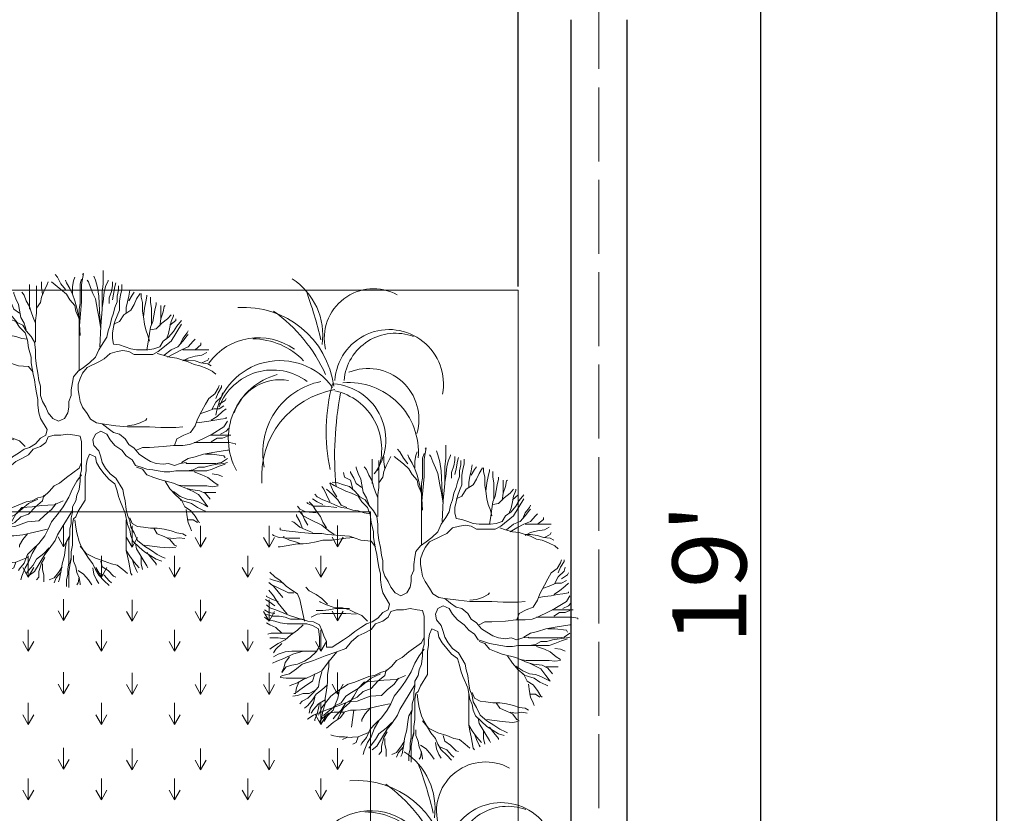
# Model space of a CAD drawing. Units: millimetres. Extents: x 595116 to 630915, y 909473 to 920225.
# Tile 111 of 134: x 629744 to 629904, y 919217 to 919346. Entities that reach past the tile are written whole.
import ezdxf

# ---------------------------------------------------------------- set-up
doc = ezdxf.new("R2010")
doc.units = ezdxf.units.MM
doc.linetypes.add('ACAD_ISO02W100', pattern=[15, 12, -3])
for name, color, linetype, lineweight in [('C-PROP', 7, 'Continuous', 25), ('C-PROP-REF', 240, 'ACAD_ISO02W100', 13), ('Dimension', 3, 'Continuous', 18), ('L-PLNT', 85, 'Continuous', 13)]:
    doc.layers.add(name, color=color, linetype=linetype, lineweight=lineweight)
doc.styles.get("Standard").update_dxf_attribs({"font": 'arial.ttf'})
doc.dimstyles.new('ISO-25', dxfattribs={"dimtxt": 9, "dimasz": 6, "dimexe": 1.25, "dimexo": 0.625, "dimtad": 1, "dimlunit": 4, "dimtxsty": 'Standard', "dimcen": 2.5, "dimadec": 0, "dimazin": 0, "dimtfac": 1, "dimtmove": 0, "dimatfit": 3, "dimfxl": 1, "dimarcsym": 0})

# ---------------------------------------------------------------- blocks, each defined once
blk = doc.blocks.new('tree')
for centre, radius, start, end in [((629595.141, 919296.95), 5.184, 352.03203, 57.07138), ((629569.835, 919289.496), 31.168, 13.14902, 20.50764), ((629604.232, 919296.737), 3.791, 61.13475, 193.10801), ((629594.259, 919292.132), 6.965, 7.40006, 94.00585), ((629589.446, 919288.922), 12.167, 24.2477, 54.37264), ((629605.429, 919293.205), 4.185, 348.99772, 176.315), ((629605.915, 919293.144), 3.963, 69.38448, 175.23101), ((629595.377, 919292.044), 4.722, 54.24842, 144.21671), ((629594.88, 919291.171), 5.506, 43.86717, 89.48049), ((629597.025, 919289.989), 5.01, 36.05808, 170.65417), ((629596.464, 919289.874), 4.4, 52.90738, 159.34709), ((629598.153, 919288.998), 5.103, 105.35763, 208.89728), ((629603.809, 919290.469), 3.92, 343.88599, 112.26625), ((629597.068, 919289.758), 3.768, 80.48165, 161.06642), ((629601.247, 919287.941), 5.545, 101.04188, 191.86923), ((629614.329, 919289.554), 13.748, 164.59254, 192.32305), ((629600.849, 919288.894), 4.324, 322.54615, 85.80496), ((629602.329, 919287.957), 5.355, 355.21411, 94.82173), ((629602.391, 919286.088), 6.769, 99.68104, 184.5451), ((629626.813, 919287.645), 25.579, 169.07531, 185.28887), ((629600.275, 919288.191), 4.585, 338.7925, 77.69211)]:
    blk.add_arc(centre, radius, start, end)
blk = doc.blocks.new('A$C143125F4')
for p, q in [((2.883, 4.834), (2.883, 5.044)), ((1.898, 4.776), (1.898, 4.865)), ((1.991, 4.82), (2.008, 4.865)), ((2.21, 4.744), (2.062, 4.865)), ((2.155, 4.937), (2.117, 4.982)), ((2.21, 4.834), (2.155, 4.937)), ((2.298, 4.847), (2.281, 4.892)), ((2.391, 4.789), (2.407, 4.879)), ((2.407, 4.879), (2.429, 4.937)), ((2.516, 4.834), (2.538, 4.91)), ((2.538, 4.82), (2.571, 5)), ((2.571, 5), (2.555, 4.982)), ((2.648, 4.865), (2.626, 4.892)), ((2.681, 4.776), (2.648, 4.865)), ((2.757, 4.892), (2.735, 4.955)), ((2.79, 4.776), (2.757, 4.892)), ((2.921, 4.789), (2.96, 4.879)), ((2.96, 4.879), (2.96, 4.892)), ((3.031, 4.802), (3.031, 4.865)), ((1.461, 4.681), (1.461, 4.699)), ((1.625, 4.655), (1.586, 4.699)), ((1.712, 4.431), (1.712, 4.82)), ((1.822, 4.368), (1.822, 4.802)), ((1.915, 4.668), (1.898, 4.776)), ((1.898, 4.623), (1.937, 4.713)), ((1.937, 4.713), (1.991, 4.82)), ((2.281, 4.744), (2.21, 4.834)), ((2.298, 4.668), (2.21, 4.744)), ((2.352, 4.758), (2.298, 4.847)), ((2.391, 4.668), (2.352, 4.758)), ((2.391, 4.681), (2.391, 4.789)), ((2.516, 4.52), (2.516, 4.834)), ((2.538, 4.547), (2.538, 4.82)), ((2.719, 4.681), (2.681, 4.776)), ((2.812, 4.637), (2.79, 4.776)), ((2.867, 4.699), (2.883, 4.834)), ((2.867, 4.431), (2.867, 4.699)), ((2.883, 4.547), (2.899, 4.699)), ((2.899, 4.699), (2.921, 4.789)), ((2.976, 4.61), (3.014, 4.713)), ((3.014, 4.713), (3.031, 4.802)), ((3.047, 4.668), (3.069, 4.789)), ((3.069, 4.789), (3.085, 4.847)), ((3.102, 4.637), (3.124, 4.731)), ((3.124, 4.731), (3.124, 4.802)), ((3.156, 4.655), (3.178, 4.744)), ((3.178, 4.744), (3.178, 4.82)), ((3.288, 4.637), (3.304, 4.731)), ((3.342, 4.655), (3.375, 4.699)), ((1.275, 4.534), (1.258, 4.61)), ((1.368, 4.61), (1.368, 4.623)), ((1.422, 4.52), (1.368, 4.61)), ((1.493, 4.592), (1.461, 4.681)), ((1.532, 4.502), (1.493, 4.592)), ((1.658, 4.565), (1.625, 4.655)), ((1.712, 4.475), (1.658, 4.565)), ((1.882, 4.534), (1.898, 4.623)), ((2.352, 4.578), (2.298, 4.668)), ((2.429, 4.489), (2.352, 4.578)), ((2.429, 4.565), (2.391, 4.668)), ((2.462, 4.444), (2.429, 4.565)), ((2.5, 4.099), (2.538, 4.547)), ((2.757, 4.592), (2.719, 4.681)), ((2.79, 4.413), (2.757, 4.592)), ((2.828, 4.296), (2.812, 4.637)), ((2.867, 4.457), (2.883, 4.547)), ((2.976, 4.52), (2.976, 4.61)), ((3.031, 4.578), (3.047, 4.668)), ((3.069, 4.457), (3.102, 4.547)), ((3.102, 4.547), (3.102, 4.637)), ((3.14, 4.565), (3.156, 4.655)), ((3.14, 4.413), (3.14, 4.565)), ((3.249, 4.457), (3.266, 4.547)), ((3.266, 4.547), (3.288, 4.637)), ((3.288, 4.565), (3.342, 4.655)), ((3.375, 4.502), (3.414, 4.592)), ((3.414, 4.592), (3.468, 4.681)), ((3.485, 4.623), (3.485, 4.681)), ((3.507, 4.534), (3.485, 4.623)), ((3.539, 4.444), (3.561, 4.547)), ((3.561, 4.547), (3.578, 4.637)), ((3.578, 4.637), (3.578, 4.655)), ((3.632, 4.534), (3.632, 4.623)), ((0.946, 4.341), (0.914, 4.386)), ((1.111, 4.399), (1.039, 4.444)), ((1.056, 4.399), (1.039, 4.431)), ((1.094, 4.31), (1.056, 4.399)), ((1.078, 4.457), (1.165, 4.444)), ((1.297, 4.31), (1.111, 4.399)), ((1.165, 4.444), (1.258, 4.413)), ((1.258, 4.413), (1.351, 4.386)), ((1.368, 4.489), (1.275, 4.534)), ((1.351, 4.386), (1.439, 4.31)), ((1.406, 4.341), (1.368, 4.489)), ((1.461, 4.431), (1.422, 4.52)), ((1.548, 4.368), (1.461, 4.431)), ((1.548, 4.413), (1.532, 4.502)), ((1.57, 4.296), (1.548, 4.413)), ((1.734, 4.386), (1.712, 4.475)), ((1.767, 4.296), (1.734, 4.386)), ((1.822, 4.444), (1.882, 4.534)), ((2.445, 4.399), (2.429, 4.489)), ((2.5, 4.278), (2.445, 4.399)), ((2.484, 4.354), (2.462, 4.444)), ((2.5, 4.431), (2.516, 4.52)), ((2.5, 3.458), (2.5, 4.431)), ((2.812, 4.31), (2.79, 4.413)), ((2.845, 4.162), (2.867, 4.431)), ((3.047, 4.368), (3.069, 4.457)), ((3.102, 4.323), (3.14, 4.413)), ((3.211, 4.341), (3.321, 4.413)), ((3.249, 4.368), (3.249, 4.457)), ((3.321, 4.413), (3.375, 4.502)), ((3.507, 4.399), (3.507, 4.534)), ((3.523, 4.31), (3.507, 4.399)), ((3.523, 4.31), (3.539, 4.444)), ((3.649, 4.444), (3.632, 4.534)), ((3.649, 4.189), (3.649, 4.444)), ((3.671, 4.233), (3.704, 4.413)), ((3.704, 4.413), (3.725, 4.502)), ((3.725, 4.502), (3.725, 4.534)), ((3.797, 4.278), (3.797, 4.489)), ((3.797, 4.278), (3.835, 4.386)), ((3.835, 4.386), (3.851, 4.475)), ((3.851, 4.475), (3.868, 4.489)), ((0.837, 4.22), (0.804, 4.265)), ((0.985, 4.251), (0.946, 4.341)), ((1.078, 4.265), (0.985, 4.341)), ((1.039, 4.144), (0.985, 4.251)), ((1.165, 4.175), (1.078, 4.265)), ((1.149, 4.22), (1.094, 4.31)), ((1.384, 4.278), (1.297, 4.31)), ((1.493, 4.233), (1.384, 4.278)), ((1.439, 4.31), (1.515, 4.22)), ((1.548, 4.144), (1.493, 4.233)), ((1.625, 4.207), (1.57, 4.296)), ((1.805, 4.207), (1.767, 4.296)), ((1.805, 4.251), (1.822, 4.368)), ((1.805, 3.906), (1.805, 4.251)), ((2.5, 4.265), (2.484, 4.354)), ((2.516, 4.009), (2.5, 4.278)), ((2.828, 4.22), (2.812, 4.31)), ((2.845, 4.207), (2.828, 4.296)), ((2.992, 4.175), (3.014, 4.278)), ((3.014, 4.278), (3.047, 4.368)), ((3.047, 4.189), (3.14, 4.233)), ((3.047, 4.144), (3.069, 4.233)), ((3.069, 4.233), (3.102, 4.323)), ((3.14, 4.233), (3.211, 4.341)), ((3.539, 4.189), (3.523, 4.31)), ((3.632, 4.144), (3.671, 4.233)), ((3.78, 4.162), (3.797, 4.278)), ((3.813, 4.207), (3.906, 4.278)), ((3.906, 4.278), (3.961, 4.341)), ((3.944, 4.175), (4.037, 4.251)), ((3.944, 4.144), (3.961, 4.233)), ((3.961, 4.233), (3.999, 4.323)), ((3.999, 4.323), (3.999, 4.341)), ((4.037, 4.251), (4.037, 4.278)), ((4.125, 4.251), (4.054, 4.162)), ((0.689, 4.117), (0.673, 4.13)), ((0.782, 4.072), (0.689, 4.117)), ((0.766, 4.086), (0.711, 4.144)), ((0.837, 4.144), (0.766, 4.189)), ((0.821, 3.996), (0.766, 4.086)), ((0.93, 4.175), (0.837, 4.22)), ((0.93, 4.099), (0.837, 4.144)), ((1.039, 4.13), (0.93, 4.175)), ((1.132, 4.086), (1.039, 4.13)), ((1.22, 4.054), (1.132, 4.086)), ((1.22, 4.086), (1.165, 4.175)), ((1.313, 4.054), (1.22, 4.086)), ((1.515, 4.22), (1.603, 4.175)), ((1.641, 4.054), (1.548, 4.144)), ((1.603, 4.175), (1.658, 4.086)), ((1.658, 4.099), (1.625, 4.207)), ((1.658, 4.086), (1.734, 3.996)), ((2.5, 3.996), (2.5, 4.099)), ((2.845, 4.117), (2.828, 4.22)), ((2.828, 3.83), (2.845, 4.162)), ((2.938, 3.983), (2.96, 4.086)), ((2.96, 4.086), (2.992, 4.175)), ((3.031, 4.054), (3.047, 4.144)), ((3.561, 4.099), (3.539, 4.189)), ((3.594, 4.009), (3.561, 4.099)), ((3.594, 3.875), (3.632, 4.144)), ((3.632, 4.099), (3.725, 4.117)), ((3.725, 4.117), (3.813, 4.207)), ((3.922, 4.041), (3.944, 4.144)), ((3.961, 3.92), (4.125, 4.189)), ((4.054, 4.162), (3.999, 4.072)), ((4.218, 4.054), (4.234, 4.086)), ((0.509, 3.92), (0.509, 3.938)), ((0.563, 3.83), (0.509, 3.92)), ((0.563, 4.027), (0.525, 4.072)), ((0.602, 3.951), (0.547, 3.996)), ((0.656, 3.983), (0.563, 4.027)), ((0.618, 3.92), (0.563, 3.983)), ((0.635, 3.862), (0.602, 3.951)), ((0.728, 3.862), (0.618, 3.92)), ((0.821, 3.965), (0.656, 3.983)), ((0.968, 4.072), (0.782, 4.072)), ((0.892, 3.906), (0.821, 3.996)), ((1.149, 4.054), (0.968, 4.072)), ((1.313, 4.041), (1.22, 4.054)), ((1.406, 4.009), (1.313, 4.041)), ((1.493, 3.996), (1.406, 4.009)), ((1.586, 3.965), (1.493, 3.996)), ((1.679, 3.951), (1.586, 3.965)), ((1.679, 3.938), (1.641, 4.054)), ((1.696, 3.817), (1.679, 3.938)), ((1.734, 3.996), (1.789, 3.906)), ((2.883, 3.893), (2.938, 3.983)), ((3.031, 3.965), (3.031, 4.054)), ((3.047, 3.875), (3.031, 3.965)), ((3.616, 3.92), (3.594, 4.009)), ((3.758, 3.754), (3.961, 3.92)), ((3.835, 3.92), (3.78, 3.83)), ((3.922, 3.983), (3.835, 3.92)), ((3.89, 3.951), (3.922, 4.041)), ((3.999, 4.072), (3.922, 3.983)), ((4.07, 3.83), (4.147, 3.92)), ((4.108, 3.875), (4.147, 3.965)), ((4.147, 3.965), (4.218, 4.054)), ((4.147, 3.92), (4.218, 4.009)), ((4.218, 4.009), (4.234, 4.027)), ((4.234, 3.83), (4.311, 3.92)), ((4.311, 3.92), (4.344, 3.951)), ((0.47, 3.817), (0.438, 3.83)), ((0.563, 3.741), (0.47, 3.817)), ((0.602, 3.727), (0.563, 3.83)), ((0.689, 3.772), (0.635, 3.862)), ((0.914, 3.772), (0.728, 3.862)), ((0.93, 3.817), (0.892, 3.906)), ((1.023, 3.682), (0.914, 3.772)), ((0.985, 3.727), (0.93, 3.817)), ((1.734, 3.665), (1.696, 3.817)), ((1.789, 3.906), (1.805, 3.785)), ((1.805, 3.785), (1.805, 3.651)), ((2.757, 3.665), (2.812, 3.785)), ((2.812, 3.785), (2.883, 3.893)), ((3.14, 3.862), (3.047, 3.875)), ((3.102, 3.754), (3.195, 3.772)), ((3.233, 3.83), (3.14, 3.862)), ((3.195, 3.772), (3.288, 3.754)), ((3.321, 3.799), (3.233, 3.83)), ((3.414, 3.785), (3.321, 3.799)), ((3.594, 3.785), (3.414, 3.785)), ((3.578, 3.785), (3.594, 3.875)), ((3.687, 3.799), (3.594, 3.785)), ((3.78, 3.83), (3.687, 3.799)), ((3.851, 3.696), (3.961, 3.785)), ((3.961, 3.785), (4.07, 3.83)), ((4.015, 3.727), (4.125, 3.785)), ((4.125, 3.785), (4.234, 3.83)), ((4.147, 3.785), (4.562, 3.785)), ((4.344, 3.785), (4.437, 3.862)), ((4.437, 3.862), (4.437, 3.893)), ((0.142, 3.606), (0.126, 3.62)), ((0.235, 3.575), (0.142, 3.606)), ((0.252, 3.696), (0.252, 3.727)), ((0.345, 3.682), (0.252, 3.696)), ((0.492, 3.665), (0.345, 3.682)), ((0.58, 3.651), (0.492, 3.665)), ((0.656, 3.696), (0.563, 3.741)), ((0.766, 3.638), (0.58, 3.651)), ((0.766, 3.651), (0.656, 3.696)), ((0.914, 3.638), (0.766, 3.638)), ((1.001, 3.62), (0.914, 3.638)), ((1.204, 3.606), (1.001, 3.62)), ((1.111, 3.62), (1.023, 3.682)), ((1.351, 3.593), (1.204, 3.606)), ((1.734, 3.575), (1.734, 3.665)), ((1.805, 3.651), (1.822, 3.53)), ((2.664, 3.575), (2.757, 3.665)), ((2.812, 3.593), (2.899, 3.638)), ((2.899, 3.638), (2.992, 3.727)), ((2.992, 3.727), (3.102, 3.754)), ((3.288, 3.754), (3.375, 3.709)), ((3.375, 3.709), (3.671, 3.709)), ((3.671, 3.709), (3.758, 3.754)), ((3.742, 3.727), (3.835, 3.696)), ((3.835, 3.696), (3.944, 3.665)), ((3.906, 3.665), (4.015, 3.727)), ((3.944, 3.665), (4.054, 3.651)), ((4.054, 3.651), (4.147, 3.62)), ((4.147, 3.606), (4.234, 3.651)), ((4.147, 3.62), (4.234, 3.593)), ((4.147, 3.62), (4.234, 3.62)), ((4.234, 3.651), (4.344, 3.682)), ((4.234, 3.62), (4.344, 3.606)), ((4.344, 3.682), (4.453, 3.696)), ((4.344, 3.606), (4.437, 3.575)), ((4.453, 3.696), (4.53, 3.741)), ((4.453, 3.575), (4.546, 3.62)), ((4.546, 3.62), (4.562, 3.651)), ((0.383, 3.561), (0.235, 3.575)), ((0.306, 3.575), (0.306, 3.593)), ((0.399, 3.53), (0.306, 3.575)), ((0.438, 3.458), (0.345, 3.441)), ((0.563, 3.561), (0.383, 3.561)), ((0.492, 3.503), (0.399, 3.53)), ((0.525, 3.472), (0.438, 3.458)), ((0.58, 3.472), (0.492, 3.503)), ((0.618, 3.472), (0.525, 3.472)), ((0.711, 3.485), (0.618, 3.472)), ((0.821, 3.503), (0.711, 3.485)), ((0.93, 3.53), (0.821, 3.503)), ((1.078, 3.53), (0.93, 3.53)), ((1.297, 3.561), (1.078, 3.53)), ((1.422, 3.575), (1.297, 3.561)), ((1.532, 3.53), (1.351, 3.593)), ((1.696, 3.517), (1.532, 3.53)), ((1.767, 3.427), (1.696, 3.517)), ((1.767, 3.396), (1.734, 3.575)), ((1.822, 3.53), (1.844, 3.414)), ((2.484, 3.441), (2.571, 3.503)), ((2.555, 3.414), (2.626, 3.503)), ((2.571, 3.503), (2.664, 3.575)), ((2.626, 3.503), (2.812, 3.593)), ((4.234, 3.593), (4.327, 3.548)), ((4.327, 3.548), (4.42, 3.53)), ((4.42, 3.53), (4.53, 3.485)), ((4.437, 3.575), (4.546, 3.561)), ((4.53, 3.485), (4.617, 3.441)), ((4.546, 3.561), (4.601, 3.53)), ((0.252, 3.427), (0.219, 3.427)), ((0.345, 3.441), (0.252, 3.427)), ((1.789, 3.306), (1.767, 3.396)), ((1.805, 3.19), (1.789, 3.306)), ((1.844, 3.414), (1.86, 3.293)), ((1.86, 3.293), (1.882, 3.203)), ((2.391, 3.261), (2.407, 3.351)), ((2.407, 3.351), (2.484, 3.441)), ((2.484, 3.234), (2.516, 3.324)), ((2.516, 3.324), (2.555, 3.414)), ((4.617, 3.441), (4.672, 3.396)), ((1.822, 3.1), (1.805, 3.19)), ((1.882, 3.203), (1.882, 3.055)), ((2.374, 3.145), (2.391, 3.261)), ((2.374, 3.055), (2.374, 3.145)), ((2.484, 3.145), (2.484, 3.234)), ((2.5, 3.055), (2.484, 3.145)), ((4.655, 3.082), (4.71, 3.172)), ((4.71, 3.172), (4.727, 3.217)), ((4.71, 3.1), (4.765, 3.19)), ((4.765, 3.19), (4.765, 3.217)), ((0.164, 2.948), (0.088, 3.024)), ((1.844, 2.993), (1.822, 3.1)), ((1.844, 2.903), (1.844, 2.993)), ((1.882, 3.055), (1.915, 2.961)), ((2.336, 2.961), (2.374, 3.055)), ((2.516, 2.961), (2.5, 3.055)), ((4.508, 2.916), (4.562, 3.01)), ((4.562, 3.01), (4.655, 3.082)), ((4.672, 3.01), (4.71, 3.1)), ((4.672, 2.948), (4.765, 3.037)), ((4.727, 2.916), (4.82, 2.979)), ((4.765, 3.037), (4.781, 3.1)), ((4.82, 2.979), (4.836, 3.01)), ((0.142, 2.8), (0.071, 2.858)), ((0.109, 2.827), (0.071, 2.858)), ((0.126, 2.903), (0.088, 2.916)), ((0.197, 2.782), (0.109, 2.827)), ((0.219, 2.872), (0.126, 2.903)), ((0.252, 2.89), (0.164, 2.948)), ((0.306, 2.845), (0.219, 2.872)), ((0.345, 2.8), (0.252, 2.89)), ((1.86, 2.782), (1.844, 2.903)), ((1.915, 2.961), (1.969, 2.872)), ((1.969, 2.872), (2.008, 2.782)), ((2.32, 2.782), (2.336, 2.872)), ((2.336, 2.872), (2.336, 2.961)), ((2.555, 2.872), (2.516, 2.961)), ((2.626, 2.769), (2.555, 2.872)), ((4.453, 2.813), (4.508, 2.916)), ((4.53, 2.8), (4.639, 2.845)), ((4.617, 2.845), (4.672, 2.948)), ((4.639, 2.845), (4.727, 2.845)), ((4.727, 2.845), (4.803, 2.89)), ((4.781, 2.8), (4.836, 2.845)), ((0.142, 2.648), (0.071, 2.737)), ((0.219, 2.71), (0.142, 2.8)), ((0.383, 2.692), (0.197, 2.782)), ((0.29, 2.621), (0.219, 2.71)), ((0.438, 2.737), (0.345, 2.8)), ((0.47, 2.692), (0.383, 2.692)), ((0.525, 2.679), (0.438, 2.737)), ((0.563, 2.589), (0.525, 2.679)), ((0.711, 2.724), (0.656, 2.782)), ((0.821, 2.666), (0.711, 2.724)), ((0.914, 2.603), (0.821, 2.666)), ((1.882, 2.692), (1.86, 2.782)), ((1.991, 2.513), (1.882, 2.692)), ((2.008, 2.782), (2.079, 2.692)), ((2.079, 2.692), (2.172, 2.648)), ((2.172, 2.648), (2.265, 2.692)), ((2.265, 2.692), (2.32, 2.782)), ((2.681, 2.679), (2.626, 2.769)), ((2.774, 2.621), (2.681, 2.679)), ((3.468, 2.621), (3.561, 2.666)), ((3.561, 2.666), (3.578, 2.692)), ((4.344, 2.576), (4.382, 2.679)), ((4.382, 2.679), (4.453, 2.813)), ((4.437, 2.769), (4.53, 2.8)), ((4.562, 2.648), (4.655, 2.666)), ((4.601, 2.666), (4.694, 2.724)), ((4.655, 2.666), (4.748, 2.679)), ((4.694, 2.724), (4.781, 2.8)), ((4.748, 2.679), (4.836, 2.692)), ((4.836, 2.692), (4.836, 2.71)), ((0.071, 2.558), (0.016, 2.589)), ((0.033, 2.634), (0.033, 2.648)), ((0.126, 2.589), (0.033, 2.634)), ((0.164, 2.486), (0.071, 2.558)), ((0.219, 2.558), (0.126, 2.589)), ((0.219, 2.531), (0.142, 2.648)), ((0.361, 2.352), (0.219, 2.531)), ((0.635, 2.244), (0.563, 2.589)), ((0.892, 2.545), (0.875, 2.558)), ((0.985, 2.5), (0.892, 2.545)), ((1.001, 2.513), (0.914, 2.603)), ((1.969, 2.424), (1.991, 2.513)), ((2.867, 2.603), (2.774, 2.621)), ((2.867, 2.603), (3.085, 2.576)), ((2.96, 2.531), (2.867, 2.603)), ((3.047, 2.468), (2.96, 2.531)), ((3.085, 2.576), (3.266, 2.558)), ((3.266, 2.576), (3.375, 2.589)), ((3.266, 2.558), (3.616, 2.558)), ((3.375, 2.589), (3.468, 2.621)), ((3.616, 2.558), (3.797, 2.545)), ((3.797, 2.545), (4.037, 2.545)), ((4.037, 2.545), (4.147, 2.558)), ((4.272, 2.468), (4.344, 2.576)), ((4.365, 2.621), (4.453, 2.634)), ((4.453, 2.634), (4.562, 2.648)), ((4.617, 2.442), (4.803, 2.558)), ((4.803, 2.558), (4.858, 2.648)), ((4.836, 2.486), (4.874, 2.531)), ((0.071, 2.379), (0, 2.424)), ((0.016, 2.352), (0.126, 2.321)), ((0.088, 2.455), (0.033, 2.5)), ((0.164, 2.365), (0.071, 2.379)), ((0.181, 2.424), (0.088, 2.455)), ((0.399, 2.334), (0.181, 2.424)), ((0.837, 2.352), (0.744, 2.307)), ((0.93, 2.41), (0.821, 2.41)), ((0.93, 2.365), (0.837, 2.352)), ((1.023, 2.424), (0.93, 2.41)), ((1.297, 2.365), (0.93, 2.365)), ((1.094, 2.468), (0.985, 2.5)), ((1.132, 2.442), (1.023, 2.424)), ((1.242, 2.455), (1.094, 2.468)), ((1.351, 2.442), (1.132, 2.442)), ((1.351, 2.424), (1.242, 2.455)), ((1.461, 2.352), (1.297, 2.365)), ((1.439, 2.379), (1.351, 2.424)), ((1.548, 2.334), (1.439, 2.379)), ((1.805, 2.289), (1.882, 2.379)), ((1.882, 2.379), (1.969, 2.424)), ((2.008, 2.397), (1.969, 2.307)), ((2.101, 2.424), (2.008, 2.397)), ((2.21, 2.424), (2.101, 2.424)), ((2.32, 2.442), (2.21, 2.424)), ((2.429, 2.424), (2.32, 2.442)), ((2.516, 2.41), (2.429, 2.424)), ((2.538, 2.321), (2.516, 2.41)), ((2.757, 2.442), (2.719, 2.352)), ((2.719, 2.352), (2.735, 2.262)), ((2.845, 2.486), (2.757, 2.442)), ((2.938, 2.442), (2.845, 2.486)), ((2.992, 2.352), (2.938, 2.442)), ((3.069, 2.262), (2.992, 2.352)), ((3.14, 2.442), (3.047, 2.468)), ((3.233, 2.365), (3.14, 2.442)), ((3.288, 2.276), (3.233, 2.365)), ((4.015, 2.262), (4.054, 2.365)), ((4.054, 2.365), (4.163, 2.424)), ((4.163, 2.424), (4.272, 2.468)), ((4.344, 2.307), (4.53, 2.397)), ((4.53, 2.397), (4.617, 2.442)), ((4.584, 2.424), (4.913, 2.424)), ((4.601, 2.321), (4.694, 2.379)), ((4.694, 2.379), (4.781, 2.379)), ((4.748, 2.442), (4.836, 2.486)), ((4.781, 2.379), (4.858, 2.41)), ((0.055, 2.262), (0, 2.307)), ((0.088, 2.186), (0.033, 2.218)), ((0.164, 2.244), (0.055, 2.262)), ((0.126, 2.321), (0.235, 2.321)), ((0.252, 2.218), (0.164, 2.244)), ((0.235, 2.321), (0.328, 2.307)), ((0.361, 2.2), (0.252, 2.218)), ((0.328, 2.307), (0.416, 2.276)), ((0.673, 2.2), (0.361, 2.2)), ((0.618, 2.262), (0.399, 2.334)), ((0.416, 2.276), (0.602, 2.276)), ((0.602, 2.276), (0.689, 2.244)), ((0.766, 2.173), (0.673, 2.2)), ((0.689, 2.244), (0.782, 2.231)), ((0.782, 2.231), (0.875, 2.186)), ((1.532, 2.141), (1.625, 2.2)), ((1.641, 2.244), (1.548, 2.334)), ((1.625, 2.2), (1.712, 2.231)), ((1.767, 2.2), (1.696, 2.11)), ((1.712, 2.231), (1.805, 2.289)), ((1.882, 2.244), (1.767, 2.2)), ((1.969, 2.307), (1.882, 2.244)), ((2.538, 1.873), (2.538, 2.321)), ((2.735, 2.262), (2.812, 2.173)), ((3.178, 2.186), (3.069, 2.262)), ((3.375, 2.218), (3.288, 2.276)), ((3.452, 2.123), (3.375, 2.218)), ((3.414, 2.186), (3.507, 2.231)), ((3.507, 2.231), (3.616, 2.231)), ((3.616, 2.231), (3.835, 2.244)), ((3.835, 2.244), (3.999, 2.262)), ((3.999, 2.262), (4.147, 2.262)), ((4.147, 2.262), (4.256, 2.276)), ((4.256, 2.276), (4.344, 2.307)), ((4.327, 2.307), (4.891, 2.307)), ((4.891, 2.307), (4.984, 2.289)), ((4.984, 2.289), (4.984, 2.276)), ((0.109, 2.052), (0.055, 2.034)), ((0.181, 2.141), (0.088, 2.186)), ((0.454, 2.052), (0.109, 2.052)), ((0.274, 2.052), (0.181, 2.141)), ((0.525, 2.097), (0.416, 2.02)), ((0.618, 2.186), (0.525, 2.097)), ((0.859, 2.123), (0.766, 2.173)), ((0.875, 1.989), (0.859, 2.123)), ((0.875, 2.186), (0.914, 2.097)), ((0.914, 2.097), (0.946, 2.007)), ((1.351, 2.007), (1.439, 2.079)), ((1.439, 2.079), (1.532, 2.141)), ((1.586, 2.052), (1.493, 2.007)), ((1.696, 2.11), (1.586, 2.052)), ((2.664, 2.123), (2.626, 2.034)), ((2.757, 2.079), (2.664, 2.123)), ((2.774, 1.989), (2.757, 2.079)), ((2.812, 2.173), (2.845, 2.079)), ((2.845, 2.079), (2.867, 1.989)), ((3.249, 2.097), (3.178, 2.186)), ((3.342, 2.034), (3.249, 2.097)), ((3.539, 2.065), (3.452, 2.123)), ((3.632, 2.007), (3.539, 2.065)), ((4.125, 1.989), (4.234, 2.052)), ((4.234, 2.052), (4.344, 2.079)), ((4.344, 2.079), (4.475, 2.123)), ((4.475, 2.123), (4.655, 2.155)), ((4.508, 2.123), (4.617, 2.123)), ((4.617, 2.123), (4.803, 2.097)), ((4.655, 2.155), (4.858, 2.186)), ((4.858, 2.052), (4.765, 1.989)), ((4.803, 2.097), (4.82, 2.065)), ((4.858, 2.186), (4.874, 2.186)), ((0.219, 1.976), (0.088, 1.976)), ((0.219, 1.886), (0.126, 1.828)), ((0.274, 1.886), (0.181, 1.796)), ((0.328, 1.962), (0.219, 1.976)), ((0.328, 1.944), (0.219, 1.886)), ((0.416, 2.02), (0.328, 1.944)), ((0.875, 1.841), (0.875, 1.989)), ((0.946, 2.007), (0.985, 1.917)), ((0.985, 1.917), (0.985, 1.828)), ((1.078, 1.828), (1.165, 1.886)), ((1.165, 1.886), (1.258, 1.944)), ((1.258, 1.944), (1.351, 2.007)), ((1.384, 1.917), (1.297, 1.81)), ((1.493, 2.007), (1.384, 1.917)), ((2.5, 1.899), (2.298, 1.752)), ((2.538, 1.989), (2.5, 1.899)), ((2.626, 2.034), (2.609, 1.944)), ((2.609, 1.944), (2.609, 1.855)), ((2.828, 1.899), (2.774, 1.989)), ((2.899, 1.81), (2.828, 1.899)), ((2.867, 1.989), (2.921, 1.899)), ((2.921, 1.899), (2.992, 1.81)), ((3.397, 1.944), (3.342, 2.034)), ((3.485, 1.917), (3.397, 1.944)), ((3.414, 1.917), (3.507, 1.886)), ((3.578, 1.886), (3.485, 1.917)), ((3.507, 1.886), (3.578, 1.796)), ((3.671, 1.873), (3.578, 1.886)), ((3.725, 1.976), (3.632, 2.007)), ((3.835, 1.962), (3.725, 1.976)), ((3.922, 1.976), (3.835, 1.962)), ((4.015, 1.944), (3.922, 1.976)), ((4.108, 1.976), (4.015, 1.944)), ((4.201, 1.989), (4.108, 1.976)), ((4.201, 1.976), (4.201, 1.989)), ((4.672, 1.976), (4.201, 1.976)), ((4.311, 1.873), (4.398, 1.917)), ((4.398, 1.917), (4.491, 1.917)), ((4.491, 1.917), (4.584, 1.944)), ((4.617, 1.886), (4.53, 1.855)), ((4.584, 1.944), (4.694, 1.962)), ((4.727, 1.931), (4.617, 1.886)), ((4.765, 1.989), (4.672, 1.976)), ((4.694, 1.962), (4.803, 1.976)), ((4.82, 1.962), (4.727, 1.931)), ((4.803, 1.976), (4.858, 1.989)), ((0.126, 1.828), (0.088, 1.796)), ((0.181, 1.796), (0.142, 1.738)), ((0.328, 1.752), (0.219, 1.72)), ((0.438, 1.765), (0.328, 1.752)), ((0.837, 1.765), (0.438, 1.765)), ((0.618, 1.765), (0.454, 1.72)), ((0.728, 1.662), (0.821, 1.752)), ((0.821, 1.752), (0.875, 1.841)), ((1.149, 1.752), (0.968, 1.693)), ((0.985, 1.828), (1.078, 1.828)), ((1.149, 1.752), (1.078, 1.662)), ((1.297, 1.81), (1.149, 1.752)), ((2.298, 1.752), (2.188, 1.662)), ((2.538, 1.796), (2.462, 1.693)), ((2.516, 1.783), (2.538, 1.873)), ((2.516, 1.693), (2.516, 1.783)), ((2.609, 1.855), (2.593, 1.765)), ((2.593, 1.765), (2.593, 1.393)), ((2.976, 1.72), (2.899, 1.81)), ((2.992, 1.81), (3.085, 1.738)), ((3.085, 1.738), (3.195, 1.559)), ((3.578, 1.796), (3.687, 1.752)), ((3.758, 1.855), (3.671, 1.873)), ((3.687, 1.752), (3.78, 1.72)), ((3.851, 1.841), (3.758, 1.855)), ((3.944, 1.841), (3.851, 1.841)), ((4.037, 1.855), (3.944, 1.841)), ((4.125, 1.855), (4.037, 1.855)), ((4.53, 1.855), (4.125, 1.855)), ((4.218, 1.855), (4.311, 1.873)), ((4.327, 1.841), (4.453, 1.796)), ((4.453, 1.796), (4.546, 1.752)), ((4.546, 1.752), (4.639, 1.675)), ((4.617, 1.81), (4.71, 1.796)), ((4.71, 1.796), (4.781, 1.765)), ((0.197, 1.604), (0.126, 1.572)), ((0.219, 1.72), (0.142, 1.675)), ((0.306, 1.649), (0.197, 1.604)), ((0.454, 1.72), (0.306, 1.649)), ((0.328, 1.586), (0.306, 1.496)), ((0.399, 1.675), (0.328, 1.586)), ((0.525, 1.559), (0.635, 1.604)), ((0.782, 1.617), (0.602, 1.559)), ((0.635, 1.604), (0.728, 1.662)), ((0.968, 1.693), (0.782, 1.617)), ((1.001, 1.572), (0.914, 1.451)), ((1.078, 1.662), (1.001, 1.572)), ((1.023, 1.617), (1.023, 1.514)), ((2.101, 1.617), (2.024, 1.528)), ((2.188, 1.662), (2.101, 1.617)), ((2.391, 1.572), (2.336, 1.438)), ((2.462, 1.693), (2.391, 1.572)), ((2.5, 1.559), (2.516, 1.693)), ((3.069, 1.649), (2.976, 1.72)), ((3.102, 1.541), (3.069, 1.649)), ((3.78, 1.72), (3.999, 1.662)), ((3.868, 1.693), (3.944, 1.572)), ((3.944, 1.572), (4.037, 1.469)), ((3.999, 1.662), (4.179, 1.586)), ((4.07, 1.631), (4.163, 1.617)), ((4.163, 1.617), (4.53, 1.617)), ((4.179, 1.586), (4.272, 1.559)), ((4.218, 1.572), (4.311, 1.528)), ((4.53, 1.617), (4.617, 1.604)), ((4.617, 1.604), (4.71, 1.617)), ((4.639, 1.675), (4.71, 1.631)), ((0.274, 1.425), (0.345, 1.514)), ((0.306, 1.496), (0.274, 1.438)), ((0.345, 1.514), (0.438, 1.541)), ((0.509, 1.483), (0.399, 1.407)), ((0.438, 1.541), (0.525, 1.559)), ((0.602, 1.559), (0.509, 1.483)), ((0.914, 1.451), (0.728, 1.362)), ((0.914, 1.438), (0.875, 1.304)), ((1.023, 1.514), (1.001, 1.393)), ((1.844, 1.425), (1.751, 1.38)), ((1.937, 1.451), (1.844, 1.425)), ((1.937, 1.469), (1.915, 1.38)), ((2.024, 1.528), (1.937, 1.451)), ((2.336, 1.438), (2.243, 1.286)), ((2.445, 1.38), (2.462, 1.469)), ((2.462, 1.469), (2.5, 1.559)), ((3.124, 1.451), (3.102, 1.541)), ((3.156, 1.362), (3.124, 1.451)), ((3.195, 1.559), (3.211, 1.469)), ((3.211, 1.469), (3.233, 1.38)), ((3.999, 1.528), (4.108, 1.451)), ((4.037, 1.469), (4.125, 1.393)), ((4.108, 1.451), (4.218, 1.407)), ((4.272, 1.559), (4.42, 1.541)), ((4.311, 1.528), (4.398, 1.483)), ((4.398, 1.483), (4.475, 1.38)), ((4.42, 1.541), (4.508, 1.496)), ((4.475, 1.514), (4.672, 1.514)), ((4.508, 1.496), (4.584, 1.407)), ((0.29, 1.38), (0.252, 1.362)), ((0.345, 1.335), (0.252, 1.348)), ((0.399, 1.407), (0.29, 1.38)), ((0.673, 1.335), (0.345, 1.335)), ((0.525, 1.259), (0.438, 1.227)), ((0.547, 1.272), (0.509, 1.183)), ((0.618, 1.317), (0.525, 1.259)), ((0.728, 1.362), (0.618, 1.317)), ((0.766, 1.286), (0.673, 1.227)), ((0.804, 1.407), (0.766, 1.286)), ((0.875, 1.304), (0.859, 1.196)), ((1.001, 1.272), (0.985, 1.138)), ((1.001, 1.393), (1.001, 1.272)), ((1.439, 1.272), (1.329, 1.241)), ((1.658, 1.362), (1.439, 1.272)), ((1.696, 1.335), (1.493, 1.169)), ((1.586, 1.272), (1.493, 1.169)), ((1.751, 1.286), (1.586, 1.272)), ((1.751, 1.38), (1.658, 1.362)), ((1.844, 1.407), (1.696, 1.335)), ((1.805, 1.286), (1.696, 1.169)), ((1.898, 1.304), (1.751, 1.286)), ((1.915, 1.38), (1.805, 1.286)), ((2.101, 1.317), (1.898, 1.304)), ((2.134, 1.335), (2.062, 1.241)), ((2.243, 1.38), (2.101, 1.317)), ((2.243, 1.286), (2.172, 1.183)), ((2.391, 1.286), (2.445, 1.38)), ((2.391, 1.196), (2.391, 1.286)), ((2.593, 1.393), (2.484, 1.214)), ((3.233, 1.183), (3.156, 1.362)), ((3.233, 1.38), (3.249, 1.241)), ((4.108, 1.393), (4.201, 1.362)), ((4.125, 1.393), (4.179, 1.286)), ((4.179, 1.286), (4.272, 1.227)), ((4.201, 1.362), (4.289, 1.335)), ((4.218, 1.407), (4.311, 1.393)), ((4.289, 1.335), (4.382, 1.272)), ((4.311, 1.393), (4.398, 1.362)), ((4.382, 1.272), (4.475, 1.227)), ((4.398, 1.362), (4.491, 1.317)), ((4.475, 1.38), (4.546, 1.286)), ((4.491, 1.317), (4.546, 1.286)), ((0.438, 1.227), (0.399, 1.214)), ((0.509, 1.183), (0.492, 1.093)), ((0.563, 1.151), (0.509, 1.107)), ((0.673, 1.227), (0.563, 1.151)), ((0.782, 1.107), (0.689, 1.017)), ((0.804, 1.138), (0.711, 1.093)), ((0.859, 1.196), (0.782, 1.107)), ((0.914, 1.151), (0.821, 1.08)), ((1.001, 1.227), (0.914, 1.151)), ((0.985, 1.138), (0.968, 1.017)), ((1.149, 1.124), (1.056, 1.048)), ((1.242, 1.183), (1.149, 1.124)), ((1.187, 1.124), (1.165, 1.017)), ((1.329, 1.241), (1.242, 1.183)), ((1.384, 1.107), (1.297, 1.048)), ((1.493, 1.169), (1.384, 1.107)), ((1.493, 1.169), (1.422, 1.048)), ((1.57, 1.124), (1.477, 1.035)), ((1.696, 1.169), (1.57, 1.124)), ((1.953, 1.151), (1.86, 1.062)), ((2.062, 1.241), (1.953, 1.151)), ((2.172, 1.183), (2.062, 1.048)), ((2.391, 1.227), (2.227, 0.959)), ((2.374, 1.107), (2.391, 1.196)), ((2.374, 1.017), (2.374, 1.107)), ((2.445, 1.124), (2.407, 1.093)), ((2.484, 1.214), (2.445, 1.124)), ((3.266, 1.003), (3.233, 1.183)), ((3.249, 1.241), (3.266, 1.151)), ((3.266, 1.151), (3.304, 1.062)), ((3.304, 1.107), (3.342, 1.017)), ((4.201, 1.241), (4.218, 1.124)), ((4.218, 1.124), (4.234, 1.035)), ((4.272, 1.227), (4.344, 1.138)), ((4.344, 1.138), (4.398, 1.048)), ((4.475, 1.227), (4.508, 1.214)), ((0.525, 1.062), (0.454, 1.048)), ((0.492, 1.093), (0.47, 1.093)), ((0.618, 1.093), (0.525, 1.062)), ((0.602, 0.972), (0.563, 0.927)), ((0.689, 1.017), (0.602, 0.972)), ((0.711, 1.093), (0.618, 1.093)), ((0.766, 0.99), (0.689, 0.9)), ((0.782, 0.945), (0.728, 0.856)), ((0.821, 1.08), (0.766, 0.99)), ((0.804, 1.035), (0.782, 0.945)), ((0.968, 0.99), (0.859, 0.927)), ((0.875, 0.945), (0.859, 0.856)), ((1.056, 1.048), (0.914, 0.869)), ((0.968, 1.017), (0.968, 0.927)), ((1.165, 1.017), (1.132, 0.927)), ((1.22, 0.945), (1.132, 0.9)), ((1.329, 0.959), (1.187, 0.9)), ((1.297, 1.048), (1.22, 0.945)), ((1.297, 0.945), (1.22, 0.824)), ((1.351, 0.945), (1.258, 0.856)), ((1.384, 0.99), (1.297, 0.945)), ((1.477, 0.972), (1.329, 0.959)), ((1.422, 1.048), (1.351, 0.945)), ((1.477, 1.035), (1.384, 0.99)), ((1.679, 1.048), (1.477, 0.972)), ((1.86, 1.062), (1.679, 1.048)), ((2.062, 1.048), (2.008, 0.927)), ((2.227, 0.959), (2.155, 0.838)), ((2.352, 0.927), (2.374, 1.017)), ((2.407, 1.093), (2.391, 1.003)), ((2.391, 1.003), (2.391, 0.676)), ((2.429, 1.08), (2.445, 0.959)), ((2.445, 0.959), (2.462, 0.869)), ((3.249, 1.08), (3.249, 0.587)), ((3.304, 0.914), (3.266, 1.003)), ((3.304, 1.062), (3.321, 0.959)), ((3.321, 0.959), (3.375, 0.869)), ((3.342, 1.017), (3.43, 0.972)), ((3.43, 0.972), (3.523, 0.959)), ((3.523, 0.959), (3.632, 0.945)), ((3.632, 0.945), (3.742, 0.945)), ((3.687, 0.945), (3.742, 0.856)), ((3.742, 0.945), (3.851, 0.927)), ((4.218, 1.08), (4.311, 1.08)), ((4.234, 1.035), (4.272, 0.945)), ((4.272, 0.945), (4.289, 0.9)), ((4.311, 1.08), (4.382, 1.035)), ((4.398, 1.048), (4.42, 1.035)), ((0.689, 0.9), (0.635, 0.856)), ((0.728, 0.856), (0.711, 0.779)), ((0.782, 0.838), (0.744, 0.779)), ((0.859, 0.927), (0.782, 0.838)), ((1.001, 0.838), (0.782, 0.748)), ((0.859, 0.856), (0.837, 0.766)), ((0.914, 0.869), (0.875, 0.779)), ((0.93, 0.811), (0.914, 0.721)), ((0.968, 0.927), (0.93, 0.811)), ((1.132, 0.9), (0.946, 0.748)), ((1.187, 0.9), (1.001, 0.838)), ((1.094, 0.824), (1.001, 0.735)), ((1.111, 0.793), (1.023, 0.779)), ((1.132, 0.927), (1.094, 0.824)), ((1.258, 0.793), (1.111, 0.793)), ((1.22, 0.824), (1.132, 0.735)), ((1.258, 0.856), (1.204, 0.766)), ((1.275, 0.793), (1.204, 0.703)), ((1.368, 0.824), (1.258, 0.793)), ((1.461, 0.824), (1.368, 0.824)), ((1.422, 0.824), (1.384, 0.556)), ((1.603, 0.838), (1.461, 0.824)), ((1.789, 0.883), (1.603, 0.838)), ((1.679, 0.856), (1.603, 0.766)), ((1.991, 0.927), (1.789, 0.883)), ((1.953, 0.824), (1.86, 0.703)), ((2.008, 0.927), (1.953, 0.824)), ((2.155, 0.838), (2.117, 0.748)), ((2.352, 0.824), (2.298, 0.735)), ((2.336, 0.748), (2.352, 0.838)), ((2.352, 0.838), (2.352, 0.927)), ((2.462, 0.869), (2.5, 0.735)), ((3.321, 0.824), (3.304, 0.914)), ((3.359, 0.735), (3.321, 0.824)), ((3.375, 0.869), (3.43, 0.748)), ((3.742, 0.856), (3.851, 0.811)), ((3.851, 0.927), (3.961, 0.9)), ((3.851, 0.811), (3.944, 0.766)), ((3.906, 0.793), (3.999, 0.779)), ((3.961, 0.9), (4.054, 0.869)), ((3.999, 0.779), (4.092, 0.793)), ((4.054, 0.869), (4.147, 0.856)), ((4.092, 0.793), (4.179, 0.779)), ((4.147, 0.856), (4.201, 0.824)), ((0.782, 0.748), (0.689, 0.69)), ((0.689, 0.69), (0.689, 0.676)), ((0.837, 0.766), (0.804, 0.676)), ((0.804, 0.676), (0.804, 0.659)), ((0.875, 0.779), (0.859, 0.748)), ((0.93, 0.703), (0.875, 0.645)), ((0.892, 0.632), (0.875, 0.632)), ((0.914, 0.721), (0.892, 0.632)), ((1.023, 0.779), (0.93, 0.703)), ((0.946, 0.748), (0.946, 0.735)), ((1.001, 0.735), (0.946, 0.645)), ((1.094, 0.632), (0.985, 0.542)), ((1.132, 0.735), (1.094, 0.69)), ((1.204, 0.703), (1.094, 0.632)), ((1.204, 0.766), (1.165, 0.69)), ((1.603, 0.766), (1.548, 0.676)), ((1.548, 0.676), (1.548, 0.645)), ((1.822, 0.659), (1.751, 0.542)), ((1.86, 0.703), (1.767, 0.614)), ((2.024, 0.632), (1.937, 0.542)), ((2.117, 0.748), (2.024, 0.614)), ((2.281, 0.645), (2.265, 0.511)), ((2.298, 0.735), (2.281, 0.645)), ((2.336, 0.39), (2.336, 0.748)), ((2.391, 0.676), (2.374, 0.569)), ((2.5, 0.735), (2.538, 0.645)), ((2.516, 0.659), (2.609, 0.542)), ((2.538, 0.645), (2.648, 0.466)), ((3.452, 0.645), (3.359, 0.735)), ((3.397, 0.703), (3.414, 0.614)), ((3.43, 0.748), (3.539, 0.659)), ((3.539, 0.569), (3.452, 0.645)), ((3.539, 0.676), (3.78, 0.645)), ((3.539, 0.659), (3.649, 0.587)), ((3.78, 0.645), (3.944, 0.632)), ((3.944, 0.766), (4.015, 0.676)), ((3.944, 0.632), (4.037, 0.645)), ((4.015, 0.676), (4.054, 0.659)), ((1.679, 0.479), (1.493, 0.403)), ((1.679, 0.524), (1.625, 0.39)), ((1.767, 0.614), (1.679, 0.524)), ((1.751, 0.542), (1.696, 0.403)), ((1.953, 0.524), (1.789, 0.255)), ((1.937, 0.542), (1.822, 0.452)), ((1.953, 0.479), (1.898, 0.39)), ((2.024, 0.614), (1.953, 0.524)), ((2.265, 0.511), (2.227, 0.376)), ((2.352, 0.358), (2.374, 0.479)), ((2.374, 0.479), (2.352, 0.376)), ((2.374, 0.569), (2.374, 0.452)), ((2.407, 0.511), (2.407, 0.421)), ((2.609, 0.542), (2.757, 0.466)), ((3.249, 0.587), (3.304, 0.497)), ((3.249, 0.587), (3.266, 0.497)), ((3.266, 0.497), (3.288, 0.403)), ((3.304, 0.497), (3.375, 0.403)), ((3.414, 0.614), (3.578, 0.345)), ((3.485, 0.497), (3.485, 0.376)), ((3.725, 0.452), (3.539, 0.569)), ((3.578, 0.556), (3.649, 0.466)), ((3.649, 0.587), (3.742, 0.524)), ((3.742, 0.524), (3.835, 0.479)), ((3.835, 0.479), (3.868, 0.466)), ((1.078, 0.421), (1.056, 0.435)), ((1.187, 0.403), (1.078, 0.421)), ((1.275, 0.403), (1.187, 0.403)), ((1.313, 0.39), (1.242, 0.358)), ((1.384, 0.39), (1.275, 0.403)), ((1.493, 0.403), (1.313, 0.39)), ((1.461, 0.314), (1.406, 0.287)), ((1.493, 0.403), (1.461, 0.314)), ((1.625, 0.39), (1.548, 0.3)), ((1.641, 0.314), (1.586, 0.179)), ((1.696, 0.403), (1.641, 0.314)), ((1.767, 0.358), (1.696, 0.269)), ((1.822, 0.452), (1.767, 0.358)), ((1.898, 0.39), (1.86, 0.255)), ((1.915, 0.376), (1.915, 0.287)), ((2.227, 0.332), (2.172, 0.242)), ((2.227, 0.376), (2.21, 0.242)), ((2.32, 0.3), (2.336, 0.39)), ((2.352, 0.345), (2.336, 0.255)), ((2.374, 0.452), (2.352, 0.358)), ((2.352, 0.376), (2.352, 0.345)), ((2.407, 0.421), (2.445, 0.332)), ((2.445, 0.332), (2.462, 0.242)), ((2.648, 0.466), (2.719, 0.376)), ((2.719, 0.376), (2.757, 0.287)), ((2.719, 0.314), (2.735, 0.211)), ((2.757, 0.466), (2.899, 0.421)), ((2.845, 0.421), (2.867, 0.332)), ((2.867, 0.332), (2.96, 0.269)), ((2.899, 0.421), (3.014, 0.376)), ((3.014, 0.376), (3.102, 0.358)), ((3.102, 0.358), (3.195, 0.287)), ((3.288, 0.403), (3.321, 0.224)), ((3.342, 0.452), (3.375, 0.358)), ((3.375, 0.403), (3.452, 0.314)), ((3.375, 0.358), (3.414, 0.269)), ((3.485, 0.376), (3.507, 0.287)), ((3.578, 0.345), (3.594, 0.314)), ((3.649, 0.466), (3.725, 0.376)), ((3.813, 0.421), (3.725, 0.452)), ((3.725, 0.376), (3.725, 0.358)), ((1.548, 0.3), (1.532, 0.269)), ((1.586, 0.179), (1.57, 0.121)), ((1.696, 0.269), (1.658, 0.224)), ((1.789, 0.255), (1.712, 0.197)), ((1.86, 0.166), (1.822, 0.121)), ((1.86, 0.255), (1.86, 0.166)), ((1.915, 0.287), (1.937, 0.197)), ((1.937, 0.197), (1.937, 0.09)), ((2.172, 0.242), (2.101, 0.152)), ((2.21, 0.242), (2.134, 0.152)), ((2.21, 0.255), (2.188, 0.134)), ((2.298, 0.121), (2.32, 0.211)), ((2.32, 0.211), (2.32, 0.3)), ((2.336, 0.255), (2.336, 0)), ((2.462, 0.242), (2.5, 0.152)), ((2.484, 0.269), (2.571, 0.211)), ((2.5, 0.166), (2.484, 0.076)), ((2.571, 0.211), (2.648, 0.121)), ((2.735, 0.211), (2.774, 0.121)), ((2.757, 0.287), (2.812, 0.197)), ((2.79, 0.242), (2.899, 0.197)), ((2.812, 0.197), (2.899, 0.108)), ((2.899, 0.197), (2.976, 0.108)), ((2.96, 0.269), (3.047, 0.179)), ((3.047, 0.179), (3.085, 0.166)), ((3.195, 0.287), (3.266, 0.224)), ((3.321, 0.224), (3.342, 0.197)), ((3.414, 0.269), (3.43, 0.242)), ((2.101, 0.152), (2.024, 0.121)), ((2.134, 0.152), (2.101, 0.076)), ((2.188, 0.134), (2.172, 0.09)), ((2.298, 0.018), (2.298, 0.121)), ((2.484, 0.076), (2.462, 0.045)), ((2.5, 0.152), (2.516, 0.063)), ((2.516, 0.063), (2.516, 0.045)), ((2.648, 0.121), (2.702, 0.045)), ((2.774, 0.121), (2.812, 0.063)), ((2.899, 0.108), (2.976, 0.031)), ((2.976, 0.108), (3.014, 0.076))]:
    blk.add_line(p, q)
blk = doc.blocks.new('*D123')
at = {"layer": 'Defpoints', "color": 0, "transparency": 16777216}
for p in [(629864.28, 919369.93), (629864.28, 919141.93), (629864.28, 919141.93)]:
    blk.add_point(p, dxfattribs=at)
at = {"layer": 'Dimension', "color": 0, "lineweight": -2, "transparency": 16777216}
for p, q in [((629864.91, 919369.93), (629865.53, 919369.93)), ((629864.28, 919363.93), (629864.28, 919147.93)), ((629864.91, 919141.93), (629865.53, 919141.93))]:
    blk.add_line(p, q, dxfattribs=at)
at = {"layer": 'Dimension', "color": 0, "transparency": 16777216}
for points in [[(629863.28, 919363.93), (629865.28, 919363.93), (629864.28, 919369.93)], [(629863.28, 919147.93), (629865.28, 919147.93), (629864.28, 919141.93)]]:
    blk.add_solid(points, dxfattribs=at)
at = {"layer": 'Dimension', "color": 0, "transparency": 16777216, "insert": (629857.53, 919255.93), "char_height": 12, "attachment_point": 5, "rotation": 90}
blk.add_mtext("19'", dxfattribs=at)
blk = doc.blocks.new('*D124')
at = {"layer": 'Defpoints', "color": 0, "transparency": 16777216}
for p in [(629865.75, 920084.93), (629865.75, 919141.93), (629902.57, 919141.93)]:
    blk.add_point(p, dxfattribs=at)
at = {"layer": 'Dimension', "color": 0, "lineweight": -2, "transparency": 16777216}
for p, q in [((629866.37, 920084.93), (629903.82, 920084.93)), ((629902.57, 920078.93), (629902.57, 919147.93)), ((629866.37, 919141.93), (629903.82, 919141.93))]:
    blk.add_line(p, q, dxfattribs=at)
at = {"layer": 'Dimension', "color": 0, "transparency": 16777216}
for points in [[(629901.57, 920078.93), (629903.57, 920078.93), (629902.57, 920084.93)], [(629901.57, 919147.93), (629903.57, 919147.93), (629902.57, 919141.93)]]:
    blk.add_solid(points, dxfattribs=at)
at = {"layer": 'Dimension', "color": 0, "transparency": 16777216, "insert": (629897.35, 919613.43), "char_height": 9, "attachment_point": 5, "rotation": 90}
blk.add_mtext('78\'-7"', dxfattribs=at)
blk = doc.blocks.new('LAWN-GRASS-TUFT')
blk.add_line((0.89, 3.49), (0.89, 0))
blk.add_lwpolyline([(0, 1.58), (0.89, 0), (1.78, 1.58)])
blk = doc.blocks.new('*D220')
at = {"layer": 'Defpoints', "color": 0, "transparency": 16777216}
for p in [(629824.95, 920160.76), (629511.27, 919302.01), (629824.95, 919302.01)]:
    blk.add_point(p, dxfattribs=at)
at = {"layer": 'Dimension', "color": 0, "lineweight": -2, "transparency": 16777216}
for p, q in [((629511.27, 919302.63), (629511.27, 920162.01)), ((629824.95, 919302.63), (629824.95, 920162.01)), ((629517.27, 920160.76), (629818.95, 920160.76))]:
    blk.add_line(p, q, dxfattribs=at)
at = {"layer": 'Dimension', "color": 0, "transparency": 16777216}
for points in [[(629517.27, 920161.76), (629517.27, 920159.76), (629511.27, 920160.76)], [(629818.95, 920161.76), (629818.95, 920159.76), (629824.95, 920160.76)]]:
    blk.add_solid(points, dxfattribs=at)
at = {"layer": 'Dimension', "color": 0, "transparency": 16777216, "insert": (629668.11, 920166.03), "char_height": 9, "attachment_point": 5}
blk.add_mtext('26\'-1 1/2"', dxfattribs=at)

msp = doc.modelspace()

# ---------------------------------------------------------------- linework, layer by layer
at = {"layer": 'C-PROP'}
for p, q in [((629833.541, 919150.928), (629833.541, 919345.928)), ((629842.541, 919345.928), (629842.541, 919141.928))]:
    msp.add_line(p, q, dxfattribs=at)
at = {"layer": 'C-PROP-REF'}
msp.add_line((629838.041, 920084.928), (629838.041, 919141.928), dxfattribs=at)
at = {"layer": 'L-PLNT'}
for p, q in [((629824.951, 919302.009), (629511.274, 919302.009)), ((629824.951, 919160.917), (629824.951, 919302.009)), ((629800.951, 919266.009), (629535.274, 919266.009)), ((629800.951, 919184.917), (629800.951, 919266.009))]:
    msp.add_line(p, q, dxfattribs=at)

# ---------------------------------------------------------------- block references
for name, p, xscale, yscale, zscale in [('A$C143125F4', (629728.194, 919253.739), 10.20167662382051, 10.20167662382051, 10.20167662382051), ('tree', (-697208.709, -1018297.752), 2.107689410566463, 2.107689410566463, 2.107689410566463), ('A$C143125F4', (629783.761, 919225.402), 10.20167662382051, 10.20167662382051, 10.20167662382051), ('tree', (-697190.499, -1018374.553), 2.107689410566463, 2.107689410566463, 2.107689410566463)]:
    msp.add_blockref(name, p, dxfattribs=dict(at, xscale=xscale, yscale=yscale, zscale=zscale))
for p in [(629750.277, 919260.374), (629761.391, 919260.275), (629772.505, 919260.275), (629783.619, 919260.275), (629794.733, 919260.324), (629744.542, 919255.397), (629756.415, 919255.397), (629768.288, 919255.397), (629780.161, 919255.397), (629792.034, 919255.397), (629750.277, 919248.371), (629761.391, 919248.272), (629772.505, 919248.272), (629783.619, 919248.272), (629794.733, 919248.322), (629744.542, 919243.395), (629756.415, 919243.395), (629768.288, 919243.395), (629780.161, 919243.395), (629792.034, 919243.395), (629750.277, 919236.497), (629761.391, 919236.398), (629772.505, 919236.398), (629783.619, 919236.398), (629794.733, 919236.447), (629744.542, 919231.52), (629756.415, 919231.52), (629768.288, 919231.52), (629780.161, 919231.52), (629792.034, 919231.52), (629750.277, 919224.241), (629761.391, 919224.142), (629772.505, 919224.142), (629783.619, 919224.142), (629794.733, 919224.191), (629744.542, 919219.264), (629756.415, 919219.264), (629768.288, 919219.264), (629780.161, 919219.264), (629792.034, 919219.264)]:
    msp.add_blockref('LAWN-GRASS-TUFT', p, dxfattribs=at)

# ---------------------------------------------------------------- dimensions: what is measured, and where the dimension line sits
at = {"layer": 'Dimension'}
dim = msp.add_linear_dim(base=(629824.951, 920160.756), p1=(629511.274, 919302.009), p2=(629824.951, 919302.009), dimstyle='ISO-25', override={"dimdec": 1, "dimlfac": 1, "dimrnd": 0, "dimzin": 1, "dimdsep": 46, "dimlunit": 4, "dimfrac": 2}, dxfattribs=at)
dim.commit()
dim.dimension.update_dxf_attribs({"geometry": '*D220', "text_midpoint": (629668.113, 920166.035)})
for base, p1, p2, override, picture, middle in [((629902.574, 919141.928), (629865.746, 920084.928), (629865.746, 919141.928), {"dimclrd": 0, "dimclre": 0, "dimclrt": 0}, '*D124', (629897.354, 919613.428)), ((629864.281, 919141.928), (629864.281, 919369.928), (629864.281, 919141.928), {"dimtxt": 12, "dimclrd": 0, "dimclre": 0, "dimclrt": 0}, '*D123', (629857.529, 919255.928))]:
    dim = msp.add_linear_dim(base=base, p1=p1, p2=p2, angle=90, dimstyle='ISO-25', override=override, dxfattribs=at)
    dim.commit()
    dim.dimension.update_dxf_attribs({"geometry": picture, "text_midpoint": middle})

doc.saveas('drawing.dxf')
